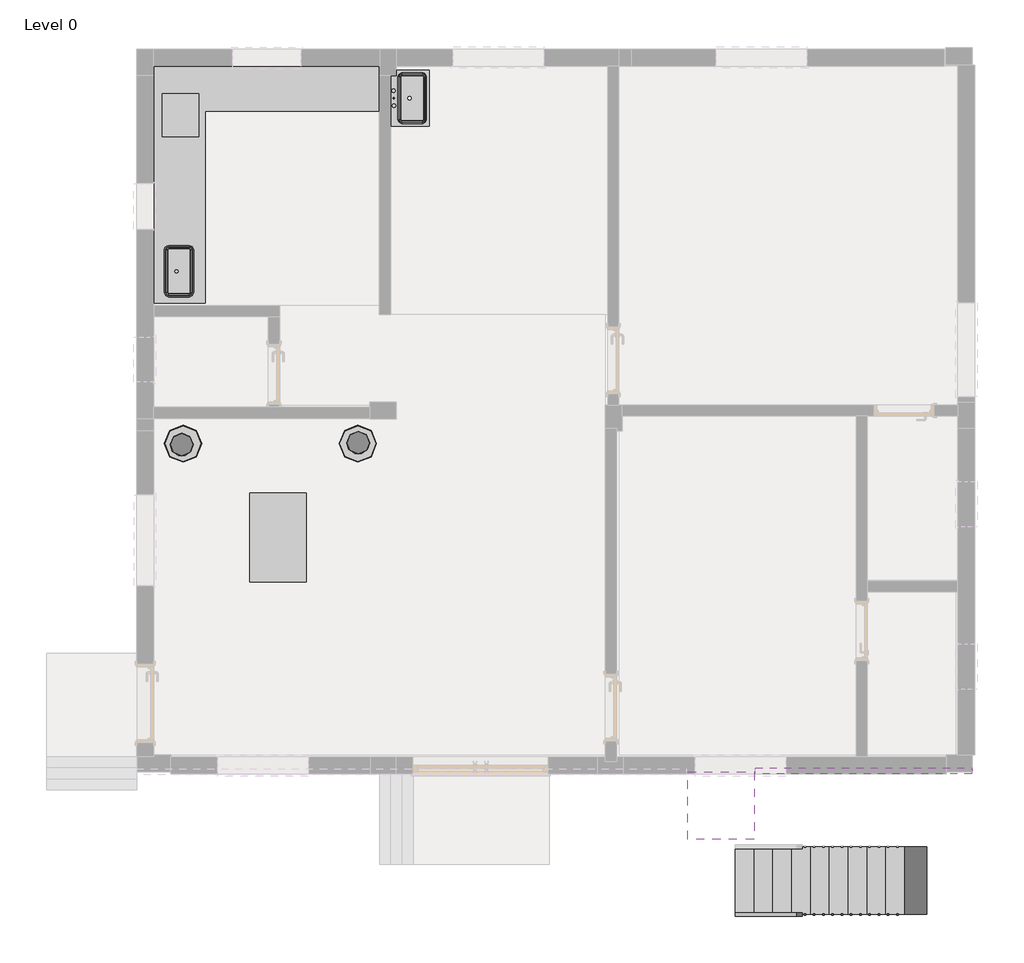
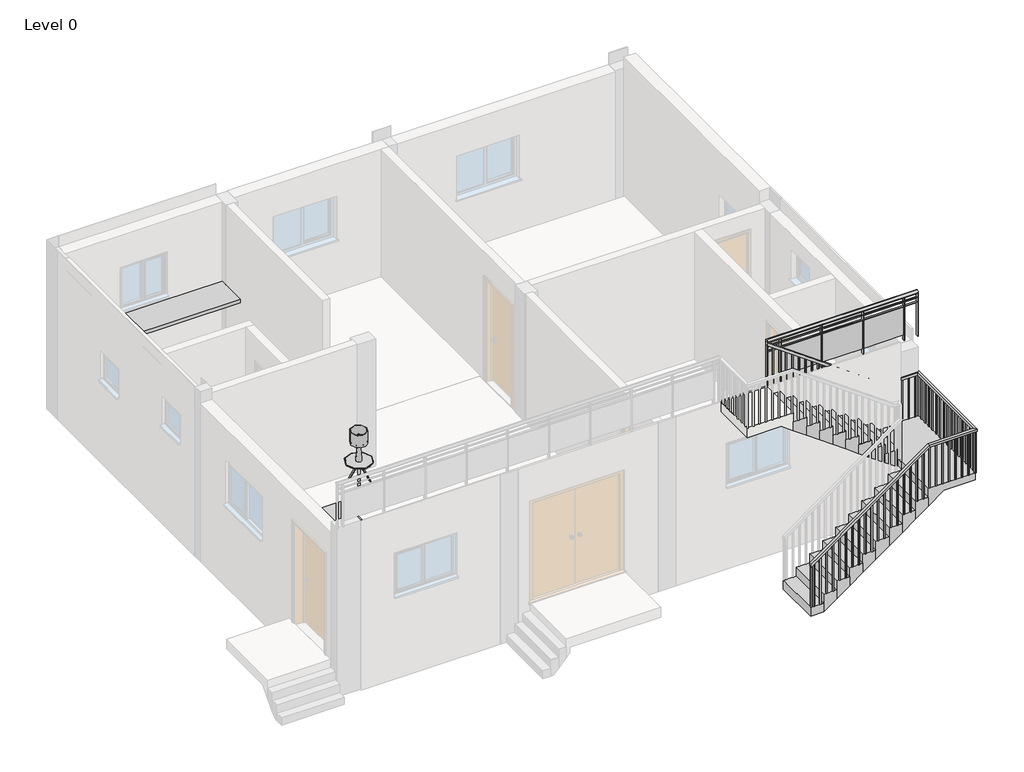
# One storey, part 3 of 3: 5 furniture elements, 2 flow terminals, 2 railings, 1 proxy, 1 slab, 1 stair flight.
"""IFC4 building model written with IfcOpenShell, lengths in millimetres."""

from ifc_helpers import new_model, si_unit, point, frame, origin, place, context, project, spatial, polyline, ellipse_curve, trimmed, outline, extrude, faceted_brep, transform, mapped, element, save
from ifc_brep_helpers import plane_surface, extruded_surface, advanced_brep
from components import generic_models_1_generic_models_1_627619a8, flow_terminal_8307eafe, furniture_2a5d2cbe, furniture_table_coffee_glass_1200x760x330mm_bccf866f, furniture_table_round_2_500mm_diameter_700mm_height_9d41381f

model = new_model("IFC4")

# Units and contexts
model_context = context("Model", 3, world=origin())
ifc_project = project(units=[si_unit("LENGTHUNIT", "METRE", prefix="MILLI")], contexts=[model_context])

# Site, building, storey
site = spatial("IfcSite", under=ifc_project)
building = spatial("IfcBuilding", under=site)
storey = spatial("IfcBuildingStorey", under=building, Name="Level 0", Elevation=0.0)

# Proxy
placement = place(None, origin())
generic_models_1_generic_models_1_shape = generic_models_1_generic_models_1_627619a8(model_context)
element("IfcBuildingElementProxy", 1, Name="Generic Models 1 : Generic Models 1", ObjectType="Generic Models 1 : Generic Models 1", at=placement, inside=storey, context=model_context, shape_type="MappedRepresentation", body=[
    mapped(generic_models_1_generic_models_1_shape, transform((0.0, 0.0, 0.0), x_axis=(1.0, 0.0, 0.0), y_axis=(0.0, 1.0, 0.0), z_axis=(0.0, 0.0, 1.0))),
])

# Flow terminals
flow_terminal_shape = flow_terminal_8307eafe(model_context)
element("IfcFlowTerminal", 2, at=placement, inside=storey, context=model_context, shape_type="MappedRepresentation", body=[
    mapped(flow_terminal_shape, transform((-6572.2460721, 7578.4046514, 149.9616), x_axis=(0.0, 1.0, 0.0), y_axis=(-1.0, 0.0, 0.0), z_axis=(0.0, 0.0, 1.0))),
])
element("IfcFlowTerminal", 3, at=placement, inside=storey, context=model_context, shape_type="MappedRepresentation", body=[
    mapped(flow_terminal_shape, transform((-9718.5420287, 5241.7332215, 458.9), x_axis=(0.0, 1.0, 0.0), y_axis=(-1.0, 0.0, 0.0), z_axis=(0.0, 0.0, 1.0))),
])

# Furniture
furniture_shape = furniture_2a5d2cbe(model_context)
element("IfcFurniture", 4, at=placement, inside=storey, context=model_context, shape_type="MappedRepresentation", body=[
    mapped(furniture_shape, transform((-9896.7493191, 2273.2763685, 609.6), x_axis=(1.0, 0.0, 0.0), y_axis=(0.0, 1.0, 0.0), z_axis=(0.0, 0.0, 1.0))),
])
element("IfcFurniture", 5, at=placement, inside=storey, context=model_context, shape_type="MappedRepresentation", body=[
    mapped(furniture_shape, transform((-7514.2898732, 2298.6763685, 609.6), x_axis=(1.0, 0.0, 0.0), y_axis=(0.0, 1.0, 0.0), z_axis=(0.0, 0.0, 1.0))),
])
furniture_table_coffee_glass_1200x760x330mm_shape = furniture_table_coffee_glass_1200x760x330mm_bccf866f(model_context)
element("IfcFurniture", 6, ObjectType="Furniture_Table_Coffee_Glass : 1200x760x330mm", at=placement, inside=storey, context=model_context, shape_type="MappedRepresentation", body=[
    mapped(furniture_table_coffee_glass_1200x760x330mm_shape, transform((-7978.1027921, 1056.4888317, 149.9616), x_axis=(0.0, 1.0, 0.0), y_axis=(-1.0, 0.0, 0.0), z_axis=(0.0, 0.0, 1.0))),
])
furniture_table_round_2_500mm_diameter_700mm_height_shape = furniture_table_round_2_500mm_diameter_700mm_height_9d41381f(model_context)
element("IfcFurniture", 7, ObjectType="Furniture_Table_Round_2 : 500mm_Diameter-700mm_Height", at=placement, inside=storey, context=model_context, shape_type="MappedRepresentation", body=[
    mapped(furniture_table_round_2_500mm_diameter_700mm_height_shape, transform((-9629.4143027, 2929.0762365, 149.9616), x_axis=(1.0, 0.0, 0.0), y_axis=(0.0, 1.0, 0.0), z_axis=(0.0, 0.0, 1.0))),
])
element("IfcFurniture", 8, ObjectType="Furniture_Table_Round_2 : 500mm_Diameter-700mm_Height", at=placement, inside=storey, context=model_context, shape_type="MappedRepresentation", body=[
    mapped(furniture_table_round_2_500mm_diameter_700mm_height_shape, transform((-7269.5415066, 2929.0762365, 149.9616), x_axis=(1.0, 0.0, 0.0), y_axis=(0.0, 1.0, 0.0), z_axis=(0.0, 0.0, 1.0))),
])

# Railings
element("IfcRailing", 9, ObjectType="900mm", at=placement, inside=storey, context=model_context, shape_type="SolidModel", body=[
    faceted_brep([(-2174.6019478, -3404.226029, 610.0312421), (-2174.6019478, -3404.226029, 548.4309995), (-2174.6019478, -3454.226029, 548.4309995), (-2174.6019478, -3454.226029, 610.0312421), (111.3425269, -3404.226029, 2255.0156211), (127.4627471, -3404.226029, 2205.0156211), (127.4627471, -3454.226029, 2205.0156211), (111.3425269, -3454.226029, 2255.0156211), (1000.7980522, -3404.226029, 2255.0156211), (1000.7980522, -3404.226029, 2205.0156211), (1050.7980522, -3454.226029, 2205.0156211), (1050.7980522, -3454.226029, 2255.0156211), (1000.7980522, -1526.447153, 2255.0156211), (1000.7980522, -1526.447153, 2205.0156211), (1050.7980522, -1476.447153, 2205.0156211), (1050.7980522, -1476.447153, 2255.0156211), (365.3355862, -1526.447153, 2255.0156211), (349.2153263, -1526.447153, 2205.0156211), (349.2153263, -1476.447153, 2205.0156211), (365.3355862, -1476.447153, 2255.0156211), (-1920.6019478, -1526.447153, 3900.0), (-1920.6019478, -1476.447153, 3900.0), (-1920.6019478, -1476.447153, 3838.3996936), (-1920.6019478, -1526.447153, 3838.3996936)], [[[0, 1, 2, 3]], [[1, 0, 4, 5]], [[2, 1, 5, 6]], [[3, 2, 6, 7]], [[0, 3, 7, 4]], [[5, 4, 8, 9]], [[6, 5, 9, 10]], [[7, 6, 10, 11]], [[4, 7, 11, 8]], [[9, 8, 12, 13]], [[10, 9, 13, 14]], [[11, 10, 14, 15]], [[8, 11, 15, 12]], [[13, 12, 16, 17]], [[14, 13, 17, 18]], [[15, 14, 18, 19]], [[12, 15, 19, 16]], [[20, 21, 22, 23]], [[17, 16, 20, 23]], [[18, 17, 23, 22]], [[19, 18, 22, 21]], [[16, 19, 21, 20]]]),
    extrude(outline(polyline([(2817.2239579, -1901.7019478), (3824.7990574, -1901.7019478), (3839.191265, -1921.7019478), (2817.2239579, -1921.7019478), (2817.2239579, -1901.7019478)])), frame((0.0, -1511.447153, 0.0), z_axis=(0.0, 1.0, 0.0), x_axis=(0.0, 0.0, 1.0)), (0.0, 0.0, 1.0), 20.0),
    extrude(outline(polyline([(2817.2239579, -1776.7019478), (3734.8477598, -1776.7019478), (3749.2399674, -1796.7019478), (2817.2239579, -1796.7019478), (2817.2239579, -1776.7019478)])), frame((0.0, -1511.447153, 0.0), z_axis=(0.0, 1.0, 0.0), x_axis=(0.0, 0.0, 1.0)), (0.0, 0.0, 1.0), 20.0),
    extrude(outline(polyline([(2634.4479158, -1651.7019478), (3644.8964622, -1651.7019478), (3659.2886698, -1671.7019478), (2634.4479158, -1671.7019478), (2634.4479158, -1651.7019478)])), frame((0.0, -1511.447153, 0.0), z_axis=(0.0, 1.0, 0.0), x_axis=(0.0, 0.0, 1.0)), (0.0, 0.0, 1.0), 20.0),
    extrude(outline(polyline([(2634.4479158, -1526.7019478), (3554.9451647, -1526.7019478), (3569.3373723, -1546.7019478), (2634.4479158, -1546.7019478), (2634.4479158, -1526.7019478)])), frame((0.0, -1511.447153, 0.0), z_axis=(0.0, 1.0, 0.0), x_axis=(0.0, 0.0, 1.0)), (0.0, 0.0, 1.0), 20.0),
    extrude(outline(polyline([(2451.6718737, -1401.7019478), (3464.9938671, -1401.7019478), (3479.3860747, -1421.7019478), (2451.6718737, -1421.7019478), (2451.6718737, -1401.7019478)])), frame((0.0, -1511.447153, 0.0), z_axis=(0.0, 1.0, 0.0), x_axis=(0.0, 0.0, 1.0)), (0.0, 0.0, 1.0), 20.0),
    extrude(outline(polyline([(2451.6718737, -1276.7019478), (3375.0425695, -1276.7019478), (3389.4347771, -1296.7019478), (2451.6718737, -1296.7019478), (2451.6718737, -1276.7019478)])), frame((0.0, -1511.447153, 0.0), z_axis=(0.0, 1.0, 0.0), x_axis=(0.0, 0.0, 1.0)), (0.0, 0.0, 1.0), 20.0),
    extrude(outline(polyline([(2451.6718737, -1151.7019478), (3285.0912719, -1151.7019478), (3299.4834795, -1171.7019478), (2451.6718737, -1171.7019478), (2451.6718737, -1151.7019478)])), frame((0.0, -1511.447153, 0.0), z_axis=(0.0, 1.0, 0.0), x_axis=(0.0, 0.0, 1.0)), (0.0, 0.0, 1.0), 20.0),
    extrude(outline(polyline([(2268.8958316, -1026.7019478), (3195.1399743, -1026.7019478), (3209.5321819, -1046.7019478), (2268.8958316, -1046.7019478), (2268.8958316, -1026.7019478)])), frame((0.0, -1511.447153, 0.0), z_axis=(0.0, 1.0, 0.0), x_axis=(0.0, 0.0, 1.0)), (0.0, 0.0, 1.0), 20.0),
    extrude(outline(polyline([(2268.8958316, -901.7019478), (3105.1886768, -901.7019478), (3119.5808844, -921.7019478), (2268.8958316, -921.7019478), (2268.8958316, -901.7019478)])), frame((0.0, -1511.447153, 0.0), z_axis=(0.0, 1.0, 0.0), x_axis=(0.0, 0.0, 1.0)), (0.0, 0.0, 1.0), 20.0),
    extrude(outline(polyline([(2086.1197895, -776.7019478), (3015.2373792, -776.7019478), (3029.6295868, -796.7019478), (2086.1197895, -796.7019478), (2086.1197895, -776.7019478)])), frame((0.0, -1511.447153, 0.0), z_axis=(0.0, 1.0, 0.0), x_axis=(0.0, 0.0, 1.0)), (0.0, 0.0, 1.0), 20.0),
    extrude(outline(polyline([(2086.1197895, -651.7019478), (2925.2860816, -651.7019478), (2939.6782892, -671.7019478), (2086.1197895, -671.7019478), (2086.1197895, -651.7019478)])), frame((0.0, -1511.447153, 0.0), z_axis=(0.0, 1.0, 0.0), x_axis=(0.0, 0.0, 1.0)), (0.0, 0.0, 1.0), 20.0),
    extrude(outline(polyline([(1903.3437474, -526.7019478), (2835.334784, -526.7019478), (2849.7269916, -546.7019478), (1903.3437474, -546.7019478), (1903.3437474, -526.7019478)])), frame((0.0, -1511.447153, 0.0), z_axis=(0.0, 1.0, 0.0), x_axis=(0.0, 0.0, 1.0)), (0.0, 0.0, 1.0), 20.0),
    extrude(outline(polyline([(1903.3437474, -401.7019478), (2745.3834864, -401.7019478), (2759.7756941, -421.7019478), (1903.3437474, -421.7019478), (1903.3437474, -401.7019478)])), frame((0.0, -1511.447153, 0.0), z_axis=(0.0, 1.0, 0.0), x_axis=(0.0, 0.0, 1.0)), (0.0, 0.0, 1.0), 20.0),
    extrude(outline(polyline([(1720.5677053, -276.7019478), (2655.4321889, -276.7019478), (2669.8243965, -296.7019478), (1720.5677053, -296.7019478), (1720.5677053, -276.7019478)])), frame((0.0, -1511.447153, 0.0), z_axis=(0.0, 1.0, 0.0), x_axis=(0.0, 0.0, 1.0)), (0.0, 0.0, 1.0), 20.0),
    extrude(outline(polyline([(1720.5677053, -151.7019478), (2565.4808913, -151.7019478), (2579.8730989, -171.7019478), (1720.5677053, -171.7019478), (1720.5677053, -151.7019478)])), frame((0.0, -1511.447153, 0.0), z_axis=(0.0, 1.0, 0.0), x_axis=(0.0, 0.0, 1.0)), (0.0, 0.0, 1.0), 20.0),
    extrude(outline(polyline([(1537.7916632, -26.7019478), (2475.5295937, -26.7019478), (2489.9218013, -46.7019478), (1537.7916632, -46.7019478), (1537.7916632, -26.7019478)])), frame((0.0, -1511.447153, 0.0), z_axis=(0.0, 1.0, 0.0), x_axis=(0.0, 0.0, 1.0)), (0.0, 0.0, 1.0), 20.0),
    extrude(outline(polyline([(1537.7916632, 98.2980522), (2385.5782961, 98.2980522), (2399.9705037, 78.2980522), (1537.7916632, 78.2980522), (1537.7916632, 98.2980522)])), frame((0.0, -1511.447153, 0.0), z_axis=(0.0, 1.0, 0.0), x_axis=(0.0, 0.0, 1.0)), (0.0, 0.0, 1.0), 20.0),
    extrude(outline(polyline([(1355.0156211, 223.2980522), (2295.6269985, 223.2980522), (2310.0192062, 203.2980522), (1355.0156211, 203.2980522), (1355.0156211, 223.2980522)])), frame((0.0, -1511.447153, 0.0), z_axis=(0.0, 1.0, 0.0), x_axis=(0.0, 0.0, 1.0)), (0.0, 0.0, 1.0), 20.0),
    extrude(outline(polyline([(1355.0156211, 348.2980522), (2205.675701, 348.2980522), (2220.0679086, 328.2980522), (1355.0156211, 328.2980522), (1355.0156211, 348.2980522)])), frame((0.0, -1511.447153, 0.0), z_axis=(0.0, 1.0, 0.0), x_axis=(0.0, 0.0, 1.0)), (0.0, 0.0, 1.0), 20.0),
    extrude(outline(polyline([(473.2980522, -1491.447153), (473.2980522, -1511.447153), (453.2980522, -1511.447153), (453.2980522, -1491.447153), (473.2980522, -1491.447153)])), frame((0.0, 0.0, 1355.0156211), z_axis=(0.0, 0.0, 1.0), x_axis=(1.0, 0.0, 0.0)), (0.0, 0.0, 1.0), 850.0),
    extrude(outline(polyline([(598.2980522, -1491.447153), (598.2980522, -1511.447153), (578.2980522, -1511.447153), (578.2980522, -1491.447153), (598.2980522, -1491.447153)])), frame((0.0, 0.0, 1355.0156211), z_axis=(0.0, 0.0, 1.0), x_axis=(1.0, 0.0, 0.0)), (0.0, 0.0, 1.0), 850.0),
    extrude(outline(polyline([(723.2980522, -1491.447153), (723.2980522, -1511.447153), (703.2980522, -1511.447153), (703.2980522, -1491.447153), (723.2980522, -1491.447153)])), frame((0.0, 0.0, 1355.0156211), z_axis=(0.0, 0.0, 1.0), x_axis=(1.0, 0.0, 0.0)), (0.0, 0.0, 1.0), 850.0),
    extrude(outline(polyline([(848.2980522, -1491.447153), (848.2980522, -1511.447153), (828.2980522, -1511.447153), (828.2980522, -1491.447153), (848.2980522, -1491.447153)])), frame((0.0, 0.0, 1355.0156211), z_axis=(0.0, 0.0, 1.0), x_axis=(1.0, 0.0, 0.0)), (0.0, 0.0, 1.0), 850.0),
    extrude(outline(polyline([(973.2980522, -1491.447153), (973.2980522, -1511.447153), (953.2980522, -1511.447153), (953.2980522, -1491.447153), (973.2980522, -1491.447153)])), frame((0.0, 0.0, 1355.0156211), z_axis=(0.0, 0.0, 1.0), x_axis=(1.0, 0.0, 0.0)), (0.0, 0.0, 1.0), 850.0),
    extrude(outline(polyline([(1035.7980522, -1626.726029), (1015.7980522, -1626.726029), (1015.7980522, -1606.726029), (1035.7980522, -1606.726029), (1035.7980522, -1626.726029)])), frame((0.0, 0.0, 1355.0156211), z_axis=(0.0, 0.0, 1.0), x_axis=(1.0, 0.0, 0.0)), (0.0, 0.0, 1.0), 850.0),
    extrude(outline(polyline([(1035.7980522, -1751.726029), (1015.7980522, -1751.726029), (1015.7980522, -1731.726029), (1035.7980522, -1731.726029), (1035.7980522, -1751.726029)])), frame((0.0, 0.0, 1355.0156211), z_axis=(0.0, 0.0, 1.0), x_axis=(1.0, 0.0, 0.0)), (0.0, 0.0, 1.0), 850.0),
    extrude(outline(polyline([(1035.7980522, -1876.726029), (1015.7980522, -1876.726029), (1015.7980522, -1856.726029), (1035.7980522, -1856.726029), (1035.7980522, -1876.726029)])), frame((0.0, 0.0, 1355.0156211), z_axis=(0.0, 0.0, 1.0), x_axis=(1.0, 0.0, 0.0)), (0.0, 0.0, 1.0), 850.0),
    extrude(outline(polyline([(1035.7980522, -2001.726029), (1015.7980522, -2001.726029), (1015.7980522, -1981.726029), (1035.7980522, -1981.726029), (1035.7980522, -2001.726029)])), frame((0.0, 0.0, 1355.0156211), z_axis=(0.0, 0.0, 1.0), x_axis=(1.0, 0.0, 0.0)), (0.0, 0.0, 1.0), 850.0),
    extrude(outline(polyline([(1035.7980522, -2126.726029), (1015.7980522, -2126.726029), (1015.7980522, -2106.726029), (1035.7980522, -2106.726029), (1035.7980522, -2126.726029)])), frame((0.0, 0.0, 1355.0156211), z_axis=(0.0, 0.0, 1.0), x_axis=(1.0, 0.0, 0.0)), (0.0, 0.0, 1.0), 850.0),
    extrude(outline(polyline([(1035.7980522, -2251.726029), (1015.7980522, -2251.726029), (1015.7980522, -2231.726029), (1035.7980522, -2231.726029), (1035.7980522, -2251.726029)])), frame((0.0, 0.0, 1355.0156211), z_axis=(0.0, 0.0, 1.0), x_axis=(1.0, 0.0, 0.0)), (0.0, 0.0, 1.0), 850.0),
    extrude(outline(polyline([(1035.7980522, -2376.726029), (1015.7980522, -2376.726029), (1015.7980522, -2356.726029), (1035.7980522, -2356.726029), (1035.7980522, -2376.726029)])), frame((0.0, 0.0, 1355.0156211), z_axis=(0.0, 0.0, 1.0), x_axis=(1.0, 0.0, 0.0)), (0.0, 0.0, 1.0), 850.0),
    extrude(outline(polyline([(1035.7980522, -2501.726029), (1015.7980522, -2501.726029), (1015.7980522, -2481.726029), (1035.7980522, -2481.726029), (1035.7980522, -2501.726029)])), frame((0.0, 0.0, 1355.0156211), z_axis=(0.0, 0.0, 1.0), x_axis=(1.0, 0.0, 0.0)), (0.0, 0.0, 1.0), 850.0),
    extrude(outline(polyline([(1035.7980522, -2626.726029), (1015.7980522, -2626.726029), (1015.7980522, -2606.726029), (1035.7980522, -2606.726029), (1035.7980522, -2626.726029)])), frame((0.0, 0.0, 1355.0156211), z_axis=(0.0, 0.0, 1.0), x_axis=(1.0, 0.0, 0.0)), (0.0, 0.0, 1.0), 850.0),
    extrude(outline(polyline([(1035.7980522, -2751.726029), (1015.7980522, -2751.726029), (1015.7980522, -2731.726029), (1035.7980522, -2731.726029), (1035.7980522, -2751.726029)])), frame((0.0, 0.0, 1355.0156211), z_axis=(0.0, 0.0, 1.0), x_axis=(1.0, 0.0, 0.0)), (0.0, 0.0, 1.0), 850.0),
    extrude(outline(polyline([(1035.7980522, -2876.726029), (1015.7980522, -2876.726029), (1015.7980522, -2856.726029), (1035.7980522, -2856.726029), (1035.7980522, -2876.726029)])), frame((0.0, 0.0, 1355.0156211), z_axis=(0.0, 0.0, 1.0), x_axis=(1.0, 0.0, 0.0)), (0.0, 0.0, 1.0), 850.0),
    extrude(outline(polyline([(1035.7980522, -3001.726029), (1015.7980522, -3001.726029), (1015.7980522, -2981.726029), (1035.7980522, -2981.726029), (1035.7980522, -3001.726029)])), frame((0.0, 0.0, 1355.0156211), z_axis=(0.0, 0.0, 1.0), x_axis=(1.0, 0.0, 0.0)), (0.0, 0.0, 1.0), 850.0),
    extrude(outline(polyline([(1035.7980522, -3126.726029), (1015.7980522, -3126.726029), (1015.7980522, -3106.726029), (1035.7980522, -3106.726029), (1035.7980522, -3126.726029)])), frame((0.0, 0.0, 1355.0156211), z_axis=(0.0, 0.0, 1.0), x_axis=(1.0, 0.0, 0.0)), (0.0, 0.0, 1.0), 850.0),
    extrude(outline(polyline([(1035.7980522, -3251.726029), (1015.7980522, -3251.726029), (1015.7980522, -3231.726029), (1035.7980522, -3231.726029), (1035.7980522, -3251.726029)])), frame((0.0, 0.0, 1355.0156211), z_axis=(0.0, 0.0, 1.0), x_axis=(1.0, 0.0, 0.0)), (0.0, 0.0, 1.0), 850.0),
    extrude(outline(polyline([(1035.7980522, -3376.726029), (1015.7980522, -3376.726029), (1015.7980522, -3356.726029), (1035.7980522, -3356.726029), (1035.7980522, -3376.726029)])), frame((0.0, 0.0, 1355.0156211), z_axis=(0.0, 0.0, 1.0), x_axis=(1.0, 0.0, 0.0)), (0.0, 0.0, 1.0), 850.0),
    extrude(outline(polyline([(1002.8980522, -3439.226029), (1002.8980522, -3419.226029), (1022.8980522, -3419.226029), (1022.8980522, -3439.226029), (1002.8980522, -3439.226029)])), frame((0.0, 0.0, 1355.0156211), z_axis=(0.0, 0.0, 1.0), x_axis=(1.0, 0.0, 0.0)), (0.0, 0.0, 1.0), 850.0),
    extrude(outline(polyline([(877.8980522, -3439.226029), (877.8980522, -3419.226029), (897.8980522, -3419.226029), (897.8980522, -3439.226029), (877.8980522, -3439.226029)])), frame((0.0, 0.0, 1355.0156211), z_axis=(0.0, 0.0, 1.0), x_axis=(1.0, 0.0, 0.0)), (0.0, 0.0, 1.0), 850.0),
    extrude(outline(polyline([(752.8980522, -3439.226029), (752.8980522, -3419.226029), (772.8980522, -3419.226029), (772.8980522, -3439.226029), (752.8980522, -3439.226029)])), frame((0.0, 0.0, 1355.0156211), z_axis=(0.0, 0.0, 1.0), x_axis=(1.0, 0.0, 0.0)), (0.0, 0.0, 1.0), 850.0),
    extrude(outline(polyline([(627.8980522, -3439.226029), (627.8980522, -3419.226029), (647.8980522, -3419.226029), (647.8980522, -3439.226029), (627.8980522, -3439.226029)])), frame((0.0, 0.0, 1355.0156211), z_axis=(0.0, 0.0, 1.0), x_axis=(1.0, 0.0, 0.0)), (0.0, 0.0, 1.0), 850.0),
    extrude(outline(polyline([(502.8980522, -3439.226029), (502.8980522, -3419.226029), (522.8980522, -3419.226029), (522.8980522, -3439.226029), (502.8980522, -3439.226029)])), frame((0.0, 0.0, 1355.0156211), z_axis=(0.0, 0.0, 1.0), x_axis=(1.0, 0.0, 0.0)), (0.0, 0.0, 1.0), 850.0),
    extrude(outline(polyline([(377.8980522, -3439.226029), (377.8980522, -3419.226029), (397.8980522, -3419.226029), (397.8980522, -3439.226029), (377.8980522, -3439.226029)])), frame((0.0, 0.0, 1355.0156211), z_axis=(0.0, 0.0, 1.0), x_axis=(1.0, 0.0, 0.0)), (0.0, 0.0, 1.0), 850.0),
    extrude(outline(polyline([(252.8980522, -3439.226029), (252.8980522, -3419.226029), (272.8980522, -3419.226029), (272.8980522, -3439.226029), (252.8980522, -3439.226029)])), frame((0.0, 0.0, 1355.0156211), z_axis=(0.0, 0.0, 1.0), x_axis=(1.0, 0.0, 0.0)), (0.0, 0.0, 1.0), 850.0),
    extrude(outline(polyline([(127.8980522, -3439.226029), (127.8980522, -3419.226029), (147.8980522, -3419.226029), (147.8980522, -3439.226029), (127.8980522, -3439.226029)])), frame((0.0, 0.0, 1355.0156211), z_axis=(0.0, 0.0, 1.0), x_axis=(1.0, 0.0, 0.0)), (0.0, 0.0, 1.0), 850.0),
    extrude(outline(polyline([(2115.3778457, 2.8980522), (1172.2395789, 2.8980522), (1172.2395789, 22.8980522), (2129.7700096, 22.8980522), (2115.3778457, 2.8980522)])), frame((0.0, -3439.226029, 0.0), z_axis=(0.0, 1.0, 0.0), x_axis=(0.0, 0.0, 1.0)), (0.0, 0.0, 1.0), 20.0),
    extrude(outline(polyline([(2025.4268212, -122.1019478), (1172.2395789, -122.1019478), (1172.2395789, -102.1019478), (2039.8189852, -102.1019478), (2025.4268212, -122.1019478)])), frame((0.0, -3439.226029, 0.0), z_axis=(0.0, 1.0, 0.0), x_axis=(0.0, 0.0, 1.0)), (0.0, 0.0, 1.0), 20.0),
    extrude(outline(polyline([(1935.4757968, -247.1019478), (989.4635368, -247.1019478), (989.4635368, -227.1019478), (1949.8679607, -227.1019478), (1935.4757968, -247.1019478)])), frame((0.0, -3439.226029, 0.0), z_axis=(0.0, 1.0, 0.0), x_axis=(0.0, 0.0, 1.0)), (0.0, 0.0, 1.0), 20.0),
    extrude(outline(polyline([(1845.5247723, -372.1019478), (989.4635368, -372.1019478), (989.4635368, -352.1019478), (1859.9169362, -352.1019478), (1845.5247723, -372.1019478)])), frame((0.0, -3439.226029, 0.0), z_axis=(0.0, 1.0, 0.0), x_axis=(0.0, 0.0, 1.0)), (0.0, 0.0, 1.0), 20.0),
    extrude(outline(polyline([(1755.5737478, -497.1019478), (806.6874947, -497.1019478), (806.6874947, -477.1019478), (1769.9659118, -477.1019478), (1755.5737478, -497.1019478)])), frame((0.0, -3439.226029, 0.0), z_axis=(0.0, 1.0, 0.0), x_axis=(0.0, 0.0, 1.0)), (0.0, 0.0, 1.0), 20.0),
    extrude(outline(polyline([(1665.6227234, -622.1019478), (806.6874947, -622.1019478), (806.6874947, -602.1019478), (1680.0148873, -602.1019478), (1665.6227234, -622.1019478)])), frame((0.0, -3439.226029, 0.0), z_axis=(0.0, 1.0, 0.0), x_axis=(0.0, 0.0, 1.0)), (0.0, 0.0, 1.0), 20.0),
    extrude(outline(polyline([(1575.6716989, -747.1019478), (623.9114526, -747.1019478), (623.9114526, -727.1019478), (1590.0638628, -727.1019478), (1575.6716989, -747.1019478)])), frame((0.0, -3439.226029, 0.0), z_axis=(0.0, 1.0, 0.0), x_axis=(0.0, 0.0, 1.0)), (0.0, 0.0, 1.0), 20.0),
    extrude(outline(polyline([(1485.7206744, -872.1019478), (623.9114526, -872.1019478), (623.9114526, -852.1019478), (1500.1128384, -852.1019478), (1485.7206744, -872.1019478)])), frame((0.0, -3439.226029, 0.0), z_axis=(0.0, 1.0, 0.0), x_axis=(0.0, 0.0, 1.0)), (0.0, 0.0, 1.0), 20.0),
    extrude(outline(polyline([(1395.76965, -997.1019478), (441.1354105, -997.1019478), (441.1354105, -977.1019478), (1410.1618139, -977.1019478), (1395.76965, -997.1019478)])), frame((0.0, -3439.226029, 0.0), z_axis=(0.0, 1.0, 0.0), x_axis=(0.0, 0.0, 1.0)), (0.0, 0.0, 1.0), 20.0),
    extrude(outline(polyline([(1305.8186255, -1122.1019478), (441.1354105, -1122.1019478), (441.1354105, -1102.1019478), (1320.2107894, -1102.1019478), (1305.8186255, -1122.1019478)])), frame((0.0, -3439.226029, 0.0), z_axis=(0.0, 1.0, 0.0), x_axis=(0.0, 0.0, 1.0)), (0.0, 0.0, 1.0), 20.0),
    extrude(outline(polyline([(1215.867601, -1247.1019478), (258.3593684, -1247.1019478), (258.3593684, -1227.1019478), (1230.259765, -1227.1019478), (1215.867601, -1247.1019478)])), frame((0.0, -3439.226029, 0.0), z_axis=(0.0, 1.0, 0.0), x_axis=(0.0, 0.0, 1.0)), (0.0, 0.0, 1.0), 20.0),
    extrude(outline(polyline([(1125.9165766, -1372.1019478), (258.3593684, -1372.1019478), (258.3593684, -1352.1019478), (1140.3087405, -1352.1019478), (1125.9165766, -1372.1019478)])), frame((0.0, -3439.226029, 0.0), z_axis=(0.0, 1.0, 0.0), x_axis=(0.0, 0.0, 1.0)), (0.0, 0.0, 1.0), 20.0),
    extrude(outline(polyline([(1035.9655521, -1497.1019478), (75.5833263, -1497.1019478), (75.5833263, -1477.1019478), (1050.357716, -1477.1019478), (1035.9655521, -1497.1019478)])), frame((0.0, -3439.226029, 0.0), z_axis=(0.0, 1.0, 0.0), x_axis=(0.0, 0.0, 1.0)), (0.0, 0.0, 1.0), 20.0),
    extrude(outline(polyline([(946.0145276, -1622.1019478), (75.5833263, -1622.1019478), (75.5833263, -1602.1019478), (960.4066916, -1602.1019478), (946.0145276, -1622.1019478)])), frame((0.0, -3439.226029, 0.0), z_axis=(0.0, 1.0, 0.0), x_axis=(0.0, 0.0, 1.0)), (0.0, 0.0, 1.0), 20.0),
    extrude(outline(polyline([(856.0635032, -1747.1019478), (-107.1927158, -1747.1019478), (-107.1927158, -1727.1019478), (870.4556671, -1727.1019478), (856.0635032, -1747.1019478)])), frame((0.0, -3439.226029, 0.0), z_axis=(0.0, 1.0, 0.0), x_axis=(0.0, 0.0, 1.0)), (0.0, 0.0, 1.0), 20.0),
    extrude(outline(polyline([(766.1124787, -1872.1019478), (-107.1927158, -1872.1019478), (-107.1927158, -1852.1019478), (780.5046426, -1852.1019478), (766.1124787, -1872.1019478)])), frame((0.0, -3439.226029, 0.0), z_axis=(0.0, 1.0, 0.0), x_axis=(0.0, 0.0, 1.0)), (0.0, 0.0, 1.0), 20.0),
    extrude(outline(polyline([(676.1614542, -1997.1019478), (-289.9687579, -1997.1019478), (-289.9687579, -1977.1019478), (690.5536182, -1977.1019478), (676.1614542, -1997.1019478)])), frame((0.0, -3439.226029, 0.0), z_axis=(0.0, 1.0, 0.0), x_axis=(0.0, 0.0, 1.0)), (0.0, 0.0, 1.0), 20.0),
    extrude(outline(polyline([(586.2104298, -2122.1019478), (-289.9687579, -2122.1019478), (-289.9687579, -2102.1019478), (600.6025937, -2102.1019478), (586.2104298, -2122.1019478)])), frame((0.0, -3439.226029, 0.0), z_axis=(0.0, 1.0, 0.0), x_axis=(0.0, 0.0, 1.0)), (0.0, 0.0, 1.0), 20.0),
    extrude(outline(polyline([(1035.7980522, -1511.447153), (1015.7980522, -1511.447153), (1015.7980522, -1491.447153), (1035.7980522, -1491.447153), (1035.7980522, -1511.447153)])), frame((0.0, 0.0, 1355.0156211), z_axis=(0.0, 0.0, 1.0), x_axis=(1.0, 0.0, 0.0)), (0.0, 0.0, 1.0), 850.0),
    extrude(outline(polyline([(1015.7980522, -3439.226029), (1015.7980522, -3419.226029), (1035.7980522, -3419.226029), (1035.7980522, -3439.226029), (1015.7980522, -3439.226029)])), frame((0.0, 0.0, 1355.0156211), z_axis=(0.0, 0.0, 1.0), x_axis=(1.0, 0.0, 0.0)), (0.0, 0.0, 1.0), 850.0),
    extrude(outline(polyline([(2817.2239579, -1900.6019478), (3824.007486, -1900.6019478), (3838.3996936, -1920.6019478), (2817.2239579, -1920.6019478), (2817.2239579, -1900.6019478)])), frame((0.0, -1511.447153, 0.0), z_axis=(0.0, 1.0, 0.0), x_axis=(0.0, 0.0, 1.0)), (0.0, 0.0, 1.0), 20.0),
    extrude(outline(polyline([(548.4309995, -2174.6019478), (-289.9687579, -2174.6019478), (-289.9687579, -2154.6019478), (562.8231634, -2154.6019478), (548.4309995, -2174.6019478)])), frame((0.0, -3439.226029, 0.0), z_axis=(0.0, 1.0, 0.0), x_axis=(0.0, 0.0, 1.0)), (0.0, 0.0, 1.0), 20.0),
])
element("IfcRailing", 10, ObjectType="Glass_Panel-Bottom_Fill", at=placement, inside=storey, context=model_context, shape_type="SolidModel", body=[
    advanced_brep(
    [(1015.7980522, -1530.8379181, 3900.0), (1015.7980522, -1490.8379181, 3870.0), (1015.7980522, -1450.8379181, 3900.0), (1015.7980522, -1490.8379181, 3930.0), (-1905.2019478, -1530.8379181, 3900.0), (-1905.2019478, -1490.8379181, 3930.0), (-1905.2019478, -1450.8379181, 3900.0), (-1905.2019478, -1490.8379181, 3870.0)],
    [
        (0, 1, ellipse_curve(frame((1015.7980522, -1490.8379181, 3900.0), z_axis=(1.0, 0.0, 0.0), x_axis=(0.0, 1.0, 0.0)), 40.0, 30.0)),
        (1, 2, ellipse_curve(frame((1015.7980522, -1490.8379181, 3900.0), z_axis=(1.0, 0.0, 0.0), x_axis=(0.0, 1.0, 0.0)), 40.0, 30.0)),
        (2, 3, ellipse_curve(frame((1015.7980522, -1490.8379181, 3900.0), z_axis=(1.0, 0.0, 0.0), x_axis=(0.0, 1.0, 0.0)), 40.0, 30.0)),
        (3, 0, ellipse_curve(frame((1015.7980522, -1490.8379181, 3900.0), z_axis=(1.0, 0.0, 0.0), x_axis=(0.0, 1.0, 0.0)), 40.0, 30.0)),
        (4, 5, ellipse_curve(frame((-1905.2019478, -1490.8379181, 3900.0), z_axis=(-1.0, 0.0, 0.0), x_axis=(0.0, 1.0, 0.0)), 40.0, 30.0)),
        (5, 6, ellipse_curve(frame((-1905.2019478, -1490.8379181, 3900.0), z_axis=(-1.0, 0.0, 0.0), x_axis=(0.0, 1.0, 0.0)), 40.0, 30.0)),
        (6, 7, ellipse_curve(frame((-1905.2019478, -1490.8379181, 3900.0), z_axis=(-1.0, 0.0, 0.0), x_axis=(0.0, 1.0, 0.0)), 40.0, 30.0)),
        (7, 4, ellipse_curve(frame((-1905.2019478, -1490.8379181, 3900.0), z_axis=(-1.0, 0.0, 0.0), x_axis=(0.0, 1.0, 0.0)), 40.0, 30.0)),
        (0, 4),
        (7, 1),
        (6, 2),
        (5, 3),
    ],
    [
        plane_surface(frame((1015.7980522, -1490.8379181, 3900.0), z_axis=(1.0, 0.0, 0.0), x_axis=(0.0, -1.0, 0.0))),
        plane_surface(frame((-1905.2019478, -1490.8379181, 3900.0), z_axis=(-1.0, 0.0, 0.0), x_axis=(0.0, -1.0, 0.0))),
        extruded_surface(trimmed(ellipse_curve(frame((-1905.2019478, -1490.8379181, 3900.0), z_axis=(1.0, 0.0, 0.0), x_axis=(0.0, 1.0, 0.0)), 40.0, 30.0), [point((-1905.2019478, -1530.8379181, 3900.0))], [point((-1905.2019478, -1490.8379181, 3870.0))], True, "CARTESIAN"), (2921.0, 0.0, 0.0), 2921.0),
        extruded_surface(trimmed(ellipse_curve(frame((-1905.2019478, -1490.8379181, 3900.0), z_axis=(1.0, 0.0, 0.0), x_axis=(0.0, 1.0, 0.0)), 40.0, 30.0), [point((-1905.2019478, -1490.8379181, 3870.0))], [point((-1905.2019478, -1450.8379181, 3900.0))], True, "CARTESIAN"), (2921.0, 0.0, 0.0), 2921.0),
        extruded_surface(trimmed(ellipse_curve(frame((-1905.2019478, -1490.8379181, 3900.0), z_axis=(1.0, 0.0, 0.0), x_axis=(0.0, 1.0, 0.0)), 40.0, 30.0), [point((-1905.2019478, -1450.8379181, 3900.0))], [point((-1905.2019478, -1490.8379181, 3930.0))], True, "CARTESIAN"), (2921.0, 0.0, 0.0), 2921.0),
        extruded_surface(trimmed(ellipse_curve(frame((-1905.2019478, -1490.8379181, 3900.0), z_axis=(1.0, 0.0, 0.0), x_axis=(0.0, 1.0, 0.0)), 40.0, 30.0), [point((-1905.2019478, -1490.8379181, 3930.0))], [point((-1905.2019478, -1530.8379181, 3900.0))], True, "CARTESIAN"), (2921.0, 0.0, 0.0), 2921.0),
    ],
    [
        (0, [[1, 2, 3, 4]]),
        (1, [[5, 6, 7, 8]]),
        (2, [[-1, 9, -8, 10]]),
        (3, [[-2, -10, -7, 11]]),
        (4, [[-3, -11, -6, 12]]),
        (5, [[-4, -12, -5, -9]]),
    ],
),
    extrude(outline(polyline([(1015.7980522, -1481.447153), (1015.7980522, -1501.447153), (-1905.2019478, -1501.447153), (-1905.2019478, -1481.447153), (1015.7980522, -1481.447153)])), frame((0.0, 0.0, 3780.0), z_axis=(0.0, 0.0, 1.0), x_axis=(1.0, 0.0, 0.0)), (0.0, 0.0, 1.0), 20.0),
    extrude(outline(polyline([(1015.7980522, -1481.447153), (1015.7980522, -1501.447153), (-1905.2019478, -1501.447153), (-1905.2019478, -1481.447153), (1015.7980522, -1481.447153)])), frame((0.0, 0.0, 3680.0), z_axis=(0.0, 0.0, 1.0), x_axis=(1.0, 0.0, 0.0)), (0.0, 0.0, 1.0), 20.0),
    extrude(outline(polyline([(-1638.7019478, -1516.447153), (-1650.7019478, -1516.447153), (-1650.7019478, -1466.447153), (-1638.7019478, -1466.447153), (-1638.7019478, -1516.447153)])), frame((0.0, 0.0, 3000.0), z_axis=(0.0, 0.0, 1.0), x_axis=(1.0, 0.0, 0.0)), (0.0, 0.0, 1.0), 870.0),
    extrude(outline(polyline([(-844.7019478, -1489.7223429), (-1644.7019478, -1489.7223429), (-1644.7019478, -1484.7223429), (-844.7019478, -1484.7223429), (-844.7019478, -1489.7223429)])), frame((0.0, 0.0, 3100.0), z_axis=(0.0, 0.0, 1.0), x_axis=(1.0, 0.0, 0.0)), (0.0, 0.0, 1.0), 600.0),
    extrude(outline(polyline([(-838.7019478, -1516.447153), (-850.7019478, -1516.447153), (-850.7019478, -1466.447153), (-838.7019478, -1466.447153), (-838.7019478, -1516.447153)])), frame((0.0, 0.0, 3000.0), z_axis=(0.0, 0.0, 1.0), x_axis=(1.0, 0.0, 0.0)), (0.0, 0.0, 1.0), 870.0),
    extrude(outline(polyline([(-44.7019478, -1489.7223429), (-844.7019478, -1489.7223429), (-844.7019478, -1484.7223429), (-44.7019478, -1484.7223429), (-44.7019478, -1489.7223429)])), frame((0.0, 0.0, 3100.0), z_axis=(0.0, 0.0, 1.0), x_axis=(1.0, 0.0, 0.0)), (0.0, 0.0, 1.0), 600.0),
    extrude(outline(polyline([(-38.7019478, -1516.447153), (-50.7019478, -1516.447153), (-50.7019478, -1466.447153), (-38.7019478, -1466.447153), (-38.7019478, -1516.447153)])), frame((0.0, 0.0, 3000.0), z_axis=(0.0, 0.0, 1.0), x_axis=(1.0, 0.0, 0.0)), (0.0, 0.0, 1.0), 870.0),
    extrude(outline(polyline([(755.2980522, -1489.7223429), (-44.7019478, -1489.7223429), (-44.7019478, -1484.7223429), (755.2980522, -1484.7223429), (755.2980522, -1489.7223429)])), frame((0.0, 0.0, 3100.0), z_axis=(0.0, 0.0, 1.0), x_axis=(1.0, 0.0, 0.0)), (0.0, 0.0, 1.0), 600.0),
    extrude(outline(polyline([(761.2980522, -1516.447153), (749.2980522, -1516.447153), (749.2980522, -1466.447153), (761.2980522, -1466.447153), (761.2980522, -1516.447153)])), frame((0.0, 0.0, 3000.0), z_axis=(0.0, 0.0, 1.0), x_axis=(1.0, 0.0, 0.0)), (0.0, 0.0, 1.0), 870.0),
    extrude(outline(polyline([(-1897.2019478, -1516.447153), (-1909.2019478, -1516.447153), (-1909.2019478, -1466.447153), (-1897.2019478, -1466.447153), (-1897.2019478, -1516.447153)])), frame((0.0, 0.0, 3000.0), z_axis=(0.0, 0.0, 1.0), x_axis=(1.0, 0.0, 0.0)), (0.0, 0.0, 1.0), 870.0),
    extrude(outline(polyline([(1019.7980522, -1516.447153), (1007.7980522, -1516.447153), (1007.7980522, -1466.447153), (1019.7980522, -1466.447153), (1019.7980522, -1516.447153)])), frame((0.0, 0.0, 3000.0), z_axis=(0.0, 0.0, 1.0), x_axis=(1.0, 0.0, 0.0)), (0.0, 0.0, 1.0), 870.0),
])

# Slab
element("IfcSlab", 11, ObjectType="200mm_Thickness", at=placement, inside=storey, context=model_context, shape_type="SolidModel", body=[
    faceted_brep([(-1920.6019478, -2413.6043721, 2999.0), (-1920.6019478, -1501.447153, 2999.0), (-2153.4737432, -1501.447153, 2999.0), (-2813.6867445, -1501.447153, 2999.0), (-2813.6867445, -2413.6043721, 2999.0), (-2153.4737432, -2413.6043721, 2999.0), (-2813.6867445, -1501.447153, 2799.0), (-2813.6867445, -2413.6043721, 2799.0), (-1920.6019478, -2413.6043721, 2631.4230387), (-1920.6019478, -2413.6043721, 2816.2239579), (-2153.4737432, -2413.6043721, 2799.0), (-1920.6019478, -1501.447153, 2631.4230387), (-2153.4737432, -1501.447153, 2799.0)], [[[0, 1, 2, 3, 4, 5]], [[4, 3, 6, 7]], [[8, 9, 0, 5, 4, 7, 10]], [[1, 11, 12, 6, 3, 2]], [[12, 10, 7, 6]], [[1, 0, 9, 8, 11]], [[10, 12, 11, 8]]]),
    extrude(outline(polyline([(-1920.6019478, -2413.6043721), (-2813.6867445, -2413.6043721), (-2813.6867445, -1501.447153), (-1920.6019478, -1501.447153), (-1920.6019478, -2413.6043721)])), frame((0.0, 0.0, 2999.0), z_axis=(0.0, 0.0, 1.0), x_axis=(1.0, 0.0, 0.0)), (0.0, 0.0, 1.0), 1.0),
])

# Stair flight
element("IfcStairFlight", 12, ObjectType="1mm_Tread-150mm_Depth", at=placement, inside=storey, context=model_context, shape_type="SolidModel", body=[
    faceted_brep([(-1920.6019478, -2514.8095641, -290.9687579), (-2174.6019478, -2514.8095641, -290.9687579), (-2174.6019478, -3429.226029, -290.9687579), (-1920.6019478, -3429.226029, -290.9687579), (-1920.6019478, -2514.8095641, -472.7448), (-2174.6019478, -2514.8095641, -472.7448), (-2174.6019478, -3429.226029, -472.7448), (-1920.6019478, -3429.226029, -472.7448), (-1666.4027046, -2514.8095641, -108.1927158), (-1920.6019478, -2514.8095641, -108.1927158), (-1920.6019478, -3429.226029, -108.1927158), (-1666.4027046, -3429.226029, -108.1927158), (-1666.4027046, -2514.8095641, -292.8411874), (-1916.4048776, -2514.8095641, -472.7448), (-1916.4048776, -3429.226029, -472.7448), (-1666.4027046, -3429.226029, -292.8411874), (-1412.9943035, -2514.8095641, 74.5833263), (-1666.4027046, -2514.8095641, 74.5833263), (-1666.4027046, -3429.226029, 74.5833263), (-1412.9943035, -3429.226029, 74.5833263), (-1412.9943035, -2514.8095641, -110.4864251), (-1412.9943035, -3429.226029, -110.4864251), (-1158.8176558, -2514.8095641, 257.3593684), (-1412.9943035, -2514.8095641, 257.3593684), (-1412.9943035, -3429.226029, 257.3593684), (-1158.8176558, -3429.226029, 257.3593684), (-1158.8176558, -2514.8095641, 72.4211738), (-1158.8176558, -3429.226029, 72.4211738), (-650.441765, -2514.8095641, 622.9114526), (-904.6184127, -2514.8095641, 622.9114526), (-904.6184127, -3429.226029, 622.9114526), (-650.441765, -3429.226029, 622.9114526), (-650.441765, -2514.8095641, 438.2526313), (-904.6184127, -2514.8095641, 255.3450325), (-904.6184127, -2514.8095641, 440.1354105), (-904.6184127, -3429.226029, 440.1354105), (-904.6184127, -3429.226029, 255.3450325), (-650.441765, -3429.226029, 438.2526313), (-397.0333639, -2514.8095641, 805.6874947), (-650.441765, -2514.8095641, 805.6874947), (-650.441765, -3429.226029, 805.6874947), (-397.0333639, -3429.226029, 805.6874947), (-397.0333639, -2514.8095641, 620.6073936), (-397.0333639, -3429.226029, 620.6073936), (-142.8341208, -2514.8095641, 988.4635368), (-397.0333639, -2514.8095641, 988.4635368), (-397.0333639, -3429.226029, 988.4635368), (-142.8341208, -3429.226029, 988.4635368), (-142.8341208, -2514.8095641, 803.5312523), (-142.8341208, -3429.226029, 803.5312523), (111.3425269, -2514.8095641, 1171.2395789), (-142.8341208, -2514.8095641, 1171.2395789), (-142.8341208, -3429.226029, 1171.2395789), (111.3425269, -3429.226029, 1171.2395789), (111.3425269, -2514.8095641, 1204.0156211), (413.6970181, -2514.8095641, 1204.0156211), (111.3425269, -3429.226029, 986.4388511), (111.3425269, -2413.6043721, 1354.0156211), (111.3425269, -2514.8095641, 1354.0156211), (111.3425269, -3429.226029, 1354.0156211), (413.6970181, -3429.226029, 1354.0156211), (1025.7980522, -3429.226029, 1354.0156211), (1025.7980522, -1498.826029, 1354.0156211), (111.3425269, -1498.826029, 1354.0156211), (111.3425269, -2413.6043721, 1204.0156211), (413.6970181, -3429.226029, 1204.0156211), (1025.7980522, -3429.226029, 1204.0156211), (111.3425269, -2413.6043721, 1536.7916632), (111.3425269, -1498.826029, 1536.7916632), (62.981747, -1498.826029, 1536.7916632), (-142.8341208, -1498.826029, 1536.7916632), (-142.8341208, -2413.6043721, 1536.7916632), (62.981747, -2413.6043721, 1536.7916632), (-142.8341208, -2413.6043721, 1352.122856), (62.981747, -2413.6043721, 1204.0156211), (111.3425269, -1498.826029, 1204.0156211), (62.981747, -1498.826029, 1204.0156211), (-142.8341208, -1498.826029, 1352.122856), (-397.0333639, -2413.6043721, 1719.5677053), (-142.8341208, -2413.6043721, 1719.5677053), (-142.8341208, -1498.826029, 1719.5677053), (-397.0333639, -1498.826029, 1719.5677053), (-397.0333639, -2413.6043721, 1535.0472701), (-397.0333639, -1498.826029, 1535.0472701), (-650.441765, -2413.6043721, 1902.3437474), (-397.0333639, -2413.6043721, 1902.3437474), (-397.0333639, -1498.826029, 1902.3437474), (-650.441765, -1498.826029, 1902.3437474), (-650.441765, -2413.6043721, 1717.4025861), (-650.441765, -1498.826029, 1717.4025861), (-904.6297104, -2413.6043721, 2085.1197895), (-650.441765, -2413.6043721, 2085.1197895), (-650.441765, -1498.826029, 2085.1197895), (-904.6297104, -1498.826029, 2085.1197895), (-904.6297104, -2413.6043721, 1900.3188702), (-904.6297104, -1498.826029, 1900.3188702), (-1412.9943035, -2413.6043721, 2450.6718737), (-1158.8176558, -2413.6043721, 2450.6718737), (-1158.8176558, -1498.826029, 2450.6718737), (-1412.9943035, -1498.826029, 2450.6718737), (-1412.9943035, -2413.6043721, 2266.1433086), (-1158.8176558, -2413.6043721, 2083.2351544), (-1158.8176558, -2413.6043721, 2267.8958316), (-1158.8176558, -1498.826029, 2267.8958316), (-1158.8176558, -1498.826029, 2083.2351544), (-1412.9943035, -1498.826029, 2266.1433086), (-1666.4027046, -2413.6043721, 2633.4479158), (-1412.9943035, -2413.6043721, 2633.4479158), (-1412.9943035, -1498.826029, 2633.4479158), (-1666.4027046, -1498.826029, 2633.4479158), (-1666.4027046, -2413.6043721, 2448.4986245), (-1666.4027046, -1498.826029, 2448.4986245), (-1920.6019478, -2413.6043721, 2816.2239579), (-1666.4027046, -2413.6043721, 2816.2239579), (-1666.4027046, -1498.826029, 2816.2239579), (-1920.6019478, -1498.826029, 2816.2239579), (-1920.6019478, -1501.447153, 2816.2239579), (-1920.6019478, -2413.6043721, 2631.4230387), (-1920.6019478, -1498.826029, 2631.4230387), (-1920.6019478, -1501.447153, 2631.4230387), (1025.7980522, -1498.826029, 1204.0156211), (-1158.8176558, -2514.8095641, 440.1354105), (-1158.8176558, -3429.226029, 440.1354105), (-904.6297104, -2413.6043721, 2267.8958316), (-904.6297104, -1498.826029, 2267.8958316)], [[[0, 1, 2, 3]], [[1, 0, 4, 5]], [[2, 1, 5, 6]], [[3, 2, 6, 7]], [[8, 9, 10, 11]], [[4, 0, 9, 8, 12, 13]], [[0, 3, 10, 9]], [[3, 7, 14, 15, 11, 10]], [[16, 17, 18, 19]], [[17, 16, 20, 12, 8]], [[8, 11, 18, 17]], [[19, 18, 11, 15, 21]], [[22, 23, 24, 25]], [[23, 22, 26, 20, 16]], [[16, 19, 24, 23]], [[25, 24, 19, 21, 27]], [[28, 29, 30, 31]], [[29, 28, 32, 33, 34]], [[34, 35, 30, 29]], [[31, 30, 35, 36, 37]], [[38, 39, 40, 41]], [[39, 38, 42, 32, 28]], [[28, 31, 40, 39]], [[41, 40, 31, 37, 43]], [[44, 45, 46, 47]], [[45, 44, 48, 42, 38]], [[38, 41, 46, 45]], [[47, 46, 41, 43, 49]], [[50, 51, 52, 53]], [[51, 50, 54, 55, 48, 44]], [[44, 47, 52, 51]], [[53, 52, 47, 49, 56]], [[57, 58, 59, 60, 61, 62, 63]], [[58, 57, 64, 54]], [[50, 53, 59, 58, 54]], [[59, 53, 56, 65, 66, 61, 60]], [[67, 68, 69, 70, 71, 72]], [[57, 67, 72, 71, 73, 74, 64]], [[57, 63, 68, 67]], [[68, 63, 75, 76, 77, 70, 69]], [[78, 79, 80, 81]], [[79, 78, 82, 73, 71]], [[71, 70, 80, 79]], [[81, 80, 70, 77, 83]], [[84, 85, 86, 87]], [[85, 84, 88, 82, 78]], [[78, 81, 86, 85]], [[87, 86, 81, 83, 89]], [[90, 91, 92, 93]], [[91, 90, 94, 88, 84]], [[84, 87, 92, 91]], [[93, 92, 87, 89, 95]], [[96, 97, 98, 99]], [[97, 96, 100, 101, 102]], [[102, 103, 98, 97]], [[99, 98, 103, 104, 105]], [[106, 107, 108, 109]], [[107, 106, 110, 100, 96]], [[96, 99, 108, 107]], [[109, 108, 99, 105, 111]], [[112, 113, 114, 115, 116]], [[113, 112, 117, 110, 106]], [[106, 109, 114, 113]], [[115, 114, 109, 111, 118]], [[117, 112, 116, 115, 118, 119]], [[5, 4, 13, 14, 7, 6]], [[48, 55, 65, 56, 49, 43, 37, 36, 27, 21, 15, 14, 13, 12, 20, 26, 33, 32, 42]], [[65, 55, 54, 64, 74, 76, 75, 120, 66]], [[76, 74, 73, 82, 88, 94, 101, 100, 110, 117, 119, 118, 111, 105, 104, 95, 89, 83, 77]], [[34, 121, 122, 35]], [[121, 34, 33, 26, 22]], [[22, 25, 122, 121]], [[35, 122, 25, 27, 36]], [[62, 61, 66, 120]], [[63, 62, 120, 75]], [[102, 123, 124, 103]], [[123, 102, 101, 94, 90]], [[90, 93, 124, 123]], [[103, 124, 93, 95, 104]]]),
    extrude(outline(polyline([(-1920.6019478, -2514.8095641), (-1920.6019478, -3429.226029), (-2174.6019478, -3429.226029), (-2174.6019478, -2514.8095641), (-1920.6019478, -2514.8095641)])), frame((0.0, 0.0, -290.9687579), z_axis=(0.0, 0.0, 1.0), x_axis=(1.0, 0.0, 0.0)), (0.0, 0.0, 1.0), 1.0),
    extrude(outline(polyline([(-1666.4027046, -2514.8095641), (-1666.4027046, -3429.226029), (-1920.6019478, -3429.226029), (-1920.6019478, -2514.8095641), (-1666.4027046, -2514.8095641)])), frame((0.0, 0.0, -108.1927158), z_axis=(0.0, 0.0, 1.0), x_axis=(1.0, 0.0, 0.0)), (0.0, 0.0, 1.0), 1.0),
    extrude(outline(polyline([(-1412.9943035, -2514.8095641), (-1412.9943035, -3429.226029), (-1666.4027046, -3429.226029), (-1666.4027046, -2514.8095641), (-1412.9943035, -2514.8095641)])), frame((0.0, 0.0, 74.5833263), z_axis=(0.0, 0.0, 1.0), x_axis=(1.0, 0.0, 0.0)), (0.0, 0.0, 1.0), 1.0),
    extrude(outline(polyline([(-1158.8176558, -2514.8095641), (-1158.8176558, -3429.226029), (-1412.9943035, -3429.226029), (-1412.9943035, -2514.8095641), (-1158.8176558, -2514.8095641)])), frame((0.0, 0.0, 257.3593684), z_axis=(0.0, 0.0, 1.0), x_axis=(1.0, 0.0, 0.0)), (0.0, 0.0, 1.0), 1.0),
    extrude(outline(polyline([(-650.441765, -2514.8095641), (-650.441765, -3429.226029), (-904.6184127, -3429.226029), (-904.6184127, -2514.8095641), (-650.441765, -2514.8095641)])), frame((0.0, 0.0, 622.9114526), z_axis=(0.0, 0.0, 1.0), x_axis=(1.0, 0.0, 0.0)), (0.0, 0.0, 1.0), 1.0),
    extrude(outline(polyline([(-397.0333639, -2514.8095641), (-397.0333639, -3429.226029), (-650.441765, -3429.226029), (-650.441765, -2514.8095641), (-397.0333639, -2514.8095641)])), frame((0.0, 0.0, 805.6874947), z_axis=(0.0, 0.0, 1.0), x_axis=(1.0, 0.0, 0.0)), (0.0, 0.0, 1.0), 1.0),
    extrude(outline(polyline([(-142.8341208, -2514.8095641), (-142.8341208, -3429.226029), (-397.0333639, -3429.226029), (-397.0333639, -2514.8095641), (-142.8341208, -2514.8095641)])), frame((0.0, 0.0, 988.4635368), z_axis=(0.0, 0.0, 1.0), x_axis=(1.0, 0.0, 0.0)), (0.0, 0.0, 1.0), 1.0),
    extrude(outline(polyline([(111.3425269, -2514.8095641), (111.3425269, -3429.226029), (-142.8341208, -3429.226029), (-142.8341208, -2514.8095641), (111.3425269, -2514.8095641)])), frame((0.0, 0.0, 1171.2395789), z_axis=(0.0, 0.0, 1.0), x_axis=(1.0, 0.0, 0.0)), (0.0, 0.0, 1.0), 1.0),
    extrude(outline(polyline([(111.3425269, -2413.6043721), (111.3425269, -1498.826029), (1025.7980522, -1498.826029), (1025.7980522, -3429.226029), (111.3425269, -3429.226029), (111.3425269, -2514.8095641), (111.3425269, -2413.6043721)])), frame((0.0, 0.0, 1354.0156211), z_axis=(0.0, 0.0, 1.0), x_axis=(1.0, 0.0, 0.0)), (0.0, 0.0, 1.0), 1.0),
    extrude(outline(polyline([(-142.8341208, -2413.6043721), (-142.8341208, -1498.826029), (111.3425269, -1498.826029), (111.3425269, -2413.6043721), (-142.8341208, -2413.6043721)])), frame((0.0, 0.0, 1536.7916632), z_axis=(0.0, 0.0, 1.0), x_axis=(1.0, 0.0, 0.0)), (0.0, 0.0, 1.0), 1.0),
    extrude(outline(polyline([(-397.0333639, -2413.6043721), (-397.0333639, -1498.826029), (-142.8341208, -1498.826029), (-142.8341208, -2413.6043721), (-397.0333639, -2413.6043721)])), frame((0.0, 0.0, 1719.5677053), z_axis=(0.0, 0.0, 1.0), x_axis=(1.0, 0.0, 0.0)), (0.0, 0.0, 1.0), 1.0),
    extrude(outline(polyline([(-650.441765, -2413.6043721), (-650.441765, -1498.826029), (-397.0333639, -1498.826029), (-397.0333639, -2413.6043721), (-650.441765, -2413.6043721)])), frame((0.0, 0.0, 1902.3437474), z_axis=(0.0, 0.0, 1.0), x_axis=(1.0, 0.0, 0.0)), (0.0, 0.0, 1.0), 1.0),
    extrude(outline(polyline([(-904.6297104, -2413.6043721), (-904.6297104, -1498.826029), (-650.441765, -1498.826029), (-650.441765, -2413.6043721), (-904.6297104, -2413.6043721)])), frame((0.0, 0.0, 2085.1197895), z_axis=(0.0, 0.0, 1.0), x_axis=(1.0, 0.0, 0.0)), (0.0, 0.0, 1.0), 1.0),
    extrude(outline(polyline([(-1412.9943035, -2413.6043721), (-1412.9943035, -1498.826029), (-1158.8176558, -1498.826029), (-1158.8176558, -2413.6043721), (-1412.9943035, -2413.6043721)])), frame((0.0, 0.0, 2450.6718737), z_axis=(0.0, 0.0, 1.0), x_axis=(1.0, 0.0, 0.0)), (0.0, 0.0, 1.0), 1.0),
    extrude(outline(polyline([(-1666.4027046, -2413.6043721), (-1666.4027046, -1498.826029), (-1412.9943035, -1498.826029), (-1412.9943035, -2413.6043721), (-1666.4027046, -2413.6043721)])), frame((0.0, 0.0, 2633.4479158), z_axis=(0.0, 0.0, 1.0), x_axis=(1.0, 0.0, 0.0)), (0.0, 0.0, 1.0), 1.0),
    extrude(outline(polyline([(-1920.6019478, -2413.6043721), (-1920.6019478, -1498.826029), (-1666.4027046, -1498.826029), (-1666.4027046, -2413.6043721), (-1920.6019478, -2413.6043721)])), frame((0.0, 0.0, 2816.2239579), z_axis=(0.0, 0.0, 1.0), x_axis=(1.0, 0.0, 0.0)), (0.0, 0.0, 1.0), 1.0),
    extrude(outline(polyline([(-904.6184127, -2514.8095641), (-904.6184127, -3429.226029), (-1158.8176558, -3429.226029), (-1158.8176558, -2514.8095641), (-904.6184127, -2514.8095641)])), frame((0.0, 0.0, 440.1354105), z_axis=(0.0, 0.0, 1.0), x_axis=(1.0, 0.0, 0.0)), (0.0, 0.0, 1.0), 1.0),
    extrude(outline(polyline([(-1158.8176558, -2413.6043721), (-1158.8176558, -1498.826029), (-904.6297104, -1498.826029), (-904.6297104, -2413.6043721), (-1158.8176558, -2413.6043721)])), frame((0.0, 0.0, 2267.8958316), z_axis=(0.0, 0.0, 1.0), x_axis=(1.0, 0.0, 0.0)), (0.0, 0.0, 1.0), 1.0),
])

save(model, "model.ifc")

# Revit data of these elements
# Type
#   Hauteur du plan de travail = 2.952756 ft
#   Profondeur = 1.755249 ft
#   Largeur = 2.493438 ft
#   Default Elevation = 0
# Type
#   Default Elevation = 0
# Type "Furniture_Table_Coffee_Glass : 1200x760x330mm"
#   Keynote = "N"
#   Height = 1.082677 ft
#   Length = 3.937008 ft
#   Width = 2.493438 ft
#   Material Base = Metal - Chrome
#   Material Top = Glass - Clear, Grey
#   Default Elevation = 0
#   Assembly Code = ""
# Type "Furniture_Table_Round_2 : 500mm_Diameter-700mm_Height"
#   Keynote = "N"
#   Material Frame = Wood - Birch
#   Material Top = Laminate - Ivory, Matte
#   Default Elevation = 0
#   Assembly Code = ""
# Type "900mm"
#   built-in parameter 1008612 = 0.019685 (stored number, unit not read)
#   built-in parameter 1008611 = 0.019685 (stored number, unit not read)
#   built-in parameter 1008609 = 0.902231 (stored number, unit not read)
#   built-in parameter 1008604 = 0.19685 (stored number, unit not read)
#   built-in parameter 1008603 = 0.164042 (stored number, unit not read)
#   Railing Height = 2.952756 ft
#   built-in parameter 1008630 = 2
#   built-in parameter 1008610 = 2
#   built-in parameter 1008608 = 1
#   built-in parameter 1008618 = Baluster_Square : 20mm
# Type "Glass_Panel-Bottom_Fill"
#   built-in parameter 1008612 = 0.019685 (stored number, unit not read)
#   built-in parameter 1008611 = 0.019685 (stored number, unit not read)
#   built-in parameter 1008609 = 0.902231 (stored number, unit not read)
#   built-in parameter 1008604 = 0.19685 (stored number, unit not read)
#   built-in parameter 1008603 = 0.164042 (stored number, unit not read)
#   Railing Height = 2.952756 ft
#   built-in parameter 1008630 = 2
#   built-in parameter 1008610 = 2
# Element 1 (IfcBuildingElementProxy, "Generic Models 1 : Generic Models 1")
#   Phase Created = New Construction
#   Materials on its faces: "Concrete, Cast-in-Place, Gray"
# Elements 2, 3 (IfcFlowTerminal)
#   Phase Created = New Construction
# Elements 4, 5 (IfcFurniture)
#   Phase Created = New Construction
#   Materials on its faces: "Metal - Chrome Polished"
# Element 6 (IfcFurniture, "Furniture_Table_Coffee_Glass : 1200x760x330mm")
#   Phase Created = New Construction
#   Materials on its faces: "Metal - Chrome", "Glass - Clear, Grey"
# Elements 7, 8 (IfcFurniture, "Furniture_Table_Round_2 : 500mm_Diameter-700mm_Height")
#   Phase Created = New Construction
#   Materials on its faces: "Wood - Birch", "Laminate - Ivory, Matte"
# Element 9 (IfcRailing, "900mm")
#   Phase Created = New Construction
# Element 10 (IfcRailing, "Glass_Panel-Bottom_Fill")
#   Phase Created = New Construction
#   Materials on its faces: "Metal - Stainless Steel,Polished", "Glass"
# Element 11 (IfcSlab, "200mm_Thickness")
#   Phase Created = New Construction
#   Materials on its faces: "Concrete, Cast-in-Place gray"
# Element 12 (IfcStairFlight, "1mm_Tread-150mm_Depth")
#   Phase Created = New Construction
#   Materials on its faces: "Concrete, Cast-in-Place gray"
# Materials
#   "Metal - Chrome": class "Metal", colour RGB 247 247 247, transparency 0
#   "Glass - Clear, Grey": class "Glass", colour RGB 252 255 255, transparency 0.64
#   "Wood - Birch": class "Wood", colour RGB 213 164 103, transparency 0
#   "Laminate - Ivory, Matte": colour RGB 247 247 239, transparency 0
#   "Concrete, Cast-in-Place, Gray": class "Concrete", colour RGB 192 192 192, transparency 0, Description = "Cast-in-place concrete", Cost = 0
#   "Metal - Chrome Polished": class "Metal", colour RGB 247 247 247, transparency 0
#   "Metal - Stainless Steel,Polished": class "Metal", colour RGB 236 239 239, transparency 0, Cost = 0
#   "Glass": class "Glass", colour RGB 0 128 192, transparency 0.9, Description = "Soda Lime Glass", Cost = 0
#   "Concrete, Cast-in-Place gray": class "Concrete", colour RGB 192 192 192, transparency 0, Description = "Cast-in-place concrete", Cost = 0
